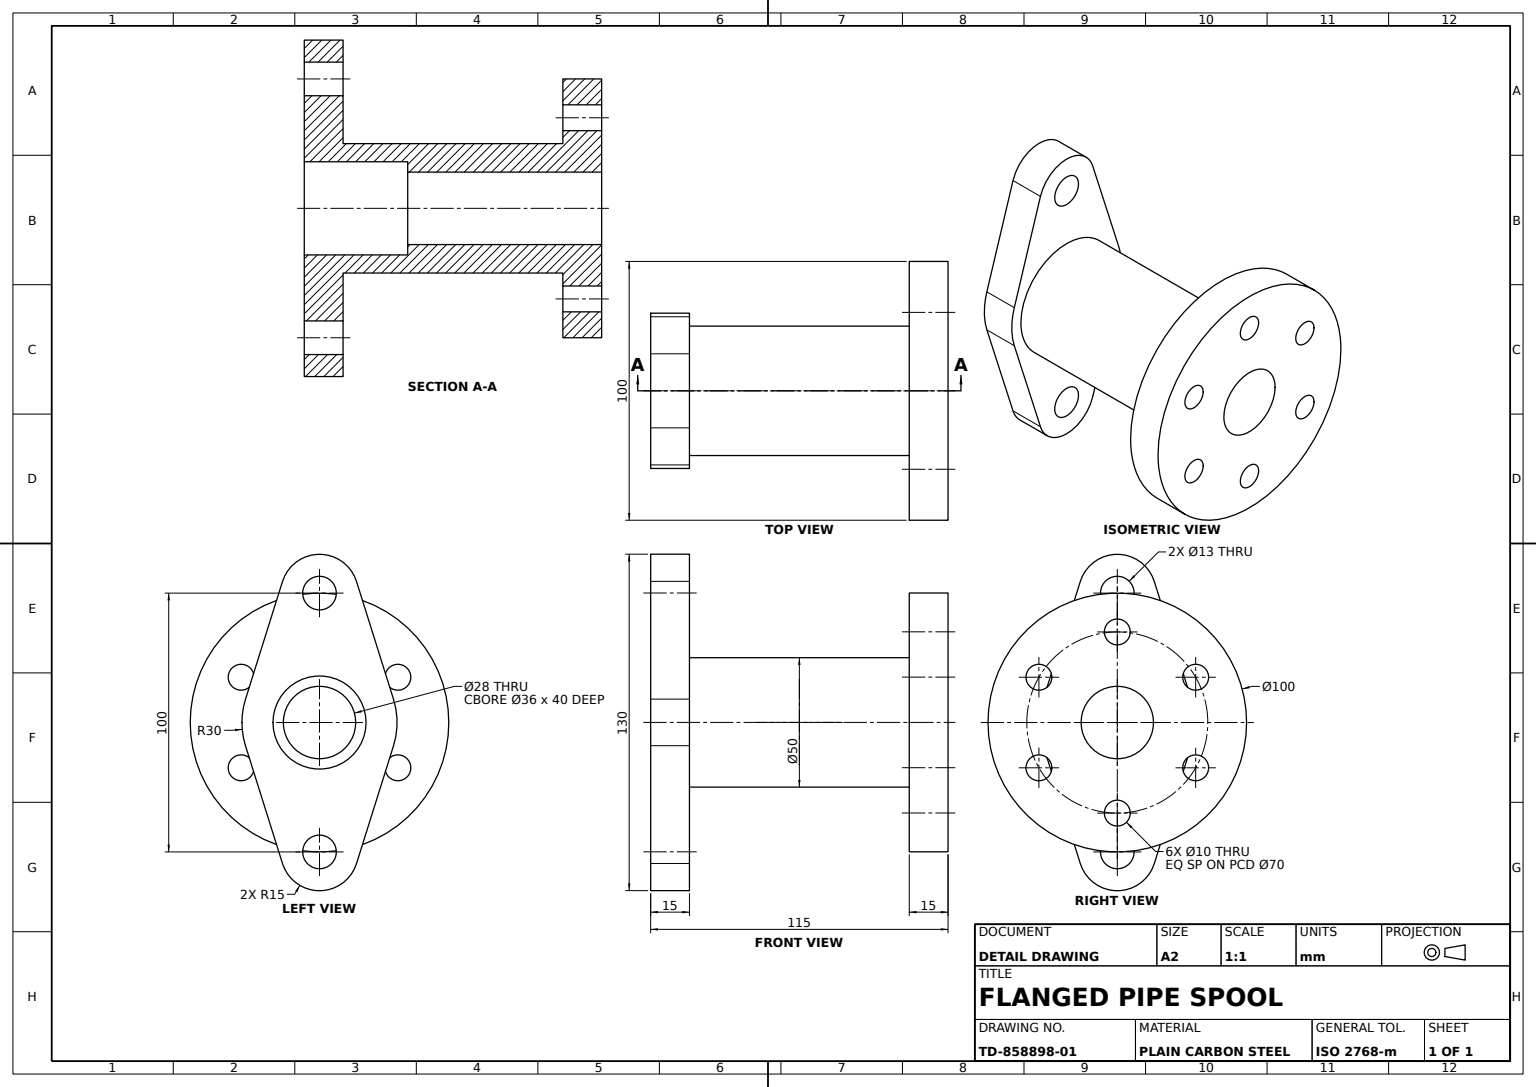
from build123d import *

# Parameters (mm, degrees)
ROUND_FLANGE_SKETCH_R            = 50
ROUND_FLANGE_100_DEPTH           = 15
ROUND_FLANGE_BOLT_HOLES_SKETCH_R = 5
ROUND_FLANGE_BOLT_HOLES_DEPTH    = 15
SPOOL_CORE_SKETCH_R              = 18
SPOOL_CORE_36_DEPTH              = 85
CORE_START                       = -85
CORE_BORE_SKETCH_R               = 18
CORE_BORE_36_DEPTH               = 85
SPOOL_PIPE_SKETCH_R              = 25
SPOOL_PIPE_50_DEPTH              = 85
OVAL_FLANGE_DEPTH                = 15
OVAL_FLANGE_HOLES_SKETCH_R       = 6.5
OVAL_FLANGE_HOLES_2X_13_DEPTH    = 15
OVAL_FLANGE_BORE_SKETCH_R        = 18
OVAL_FLANGE_BORE_36_DEPTH        = 40
THROUGH_BORE_SKETCH_R            = 14
THROUGH_BORE_28_DEPTH            = 75


with BuildPart() as part:
    # Round Flange Sketch → Round Flange Ø100 (new body)
    with BuildSketch(Plane.XY):
        Circle(ROUND_FLANGE_SKETCH_R)
    extrude(amount=ROUND_FLANGE_100_DEPTH)

    # Round Flange Bolt Holes Sketch → Round Flange Bolt Holes (cut)
    with BuildSketch(Plane.XY.offset(15)):
        with Locations((-30.310889132, 17.5)):
            Circle(ROUND_FLANGE_BOLT_HOLES_SKETCH_R)
        with Locations((0, 35)):
            Circle(ROUND_FLANGE_BOLT_HOLES_SKETCH_R)
        with Locations((30.310889132, 17.5)):
            Circle(ROUND_FLANGE_BOLT_HOLES_SKETCH_R)
        with Locations((-30.310889132, -17.5)):
            Circle(ROUND_FLANGE_BOLT_HOLES_SKETCH_R)
        with Locations((30.310889132, -17.5)):
            Circle(ROUND_FLANGE_BOLT_HOLES_SKETCH_R)
        with Locations((0, -35)):
            Circle(ROUND_FLANGE_BOLT_HOLES_SKETCH_R)
    extrude(amount=-ROUND_FLANGE_BOLT_HOLES_DEPTH, mode=Mode.SUBTRACT)

    # Spool Core Sketch → Spool Core Ø36 (add)
    with BuildSketch(Plane.XY.offset(15)):
        Circle(SPOOL_CORE_SKETCH_R)
    extrude(amount=SPOOL_CORE_36_DEPTH)

    # Core Bore Sketch → Core Bore Ø36 (cut)
    with BuildSketch(Plane.XY.offset(100).offset(CORE_START)):
        Circle(CORE_BORE_SKETCH_R)
    extrude(amount=CORE_BORE_36_DEPTH, mode=Mode.SUBTRACT)

    # Spool Pipe Sketch → Spool Pipe Ø50 (add)
    with BuildSketch(Plane.XY.offset(15)):
        Circle(SPOOL_PIPE_SKETCH_R)
    extrude(amount=SPOOL_PIPE_50_DEPTH)

    # Oval Flange Sketch → Oval Flange (add)
    with BuildSketch(Plane.XY.offset(100)):
        with BuildLine():
            Line((-28.618176043, 9), (-14.309088021, 54.5))
            ThreePointArc((-14.309088021, 54.5), (0, 65), (14.309088021, 54.5))
            Line((14.309088021, 54.5), (28.618176043, 9))
            ThreePointArc((28.618176043, 9), (30, 0), (28.618176043, -9))
            Line((28.618176043, -9), (14.309088021, -54.5))
            ThreePointArc((14.309088021, -54.5), (0, -65), (-14.309088021, -54.5))
            Line((-14.309088021, -54.5), (-28.618176043, -9))
            ThreePointArc((-28.618176043, -9), (-30, 0), (-28.618176043, 9))
        make_face()
    extrude(amount=OVAL_FLANGE_DEPTH)

    # Oval Flange Holes Sketch → Oval Flange Holes 2xØ13 (cut)
    with BuildSketch(Plane.XY.offset(115)):
        with Locations((0, 50)):
            Circle(OVAL_FLANGE_HOLES_SKETCH_R)
        with Locations((0, -50)):
            Circle(OVAL_FLANGE_HOLES_SKETCH_R)
    extrude(amount=-OVAL_FLANGE_HOLES_2X_13_DEPTH, mode=Mode.SUBTRACT)

    # Oval Flange Bore Sketch → Oval Flange Bore Ø36 (cut)
    with BuildSketch(Plane.XY.offset(115)):
        Circle(OVAL_FLANGE_BORE_SKETCH_R)
    extrude(amount=-OVAL_FLANGE_BORE_36_DEPTH, mode=Mode.SUBTRACT)

    # Through Bore Sketch → Through Bore Ø28 (cut)
    with BuildSketch(Plane.XY.offset(75)):
        Circle(THROUGH_BORE_SKETCH_R)
    extrude(amount=-THROUGH_BORE_28_DEPTH, mode=Mode.SUBTRACT)


solid = part.part
